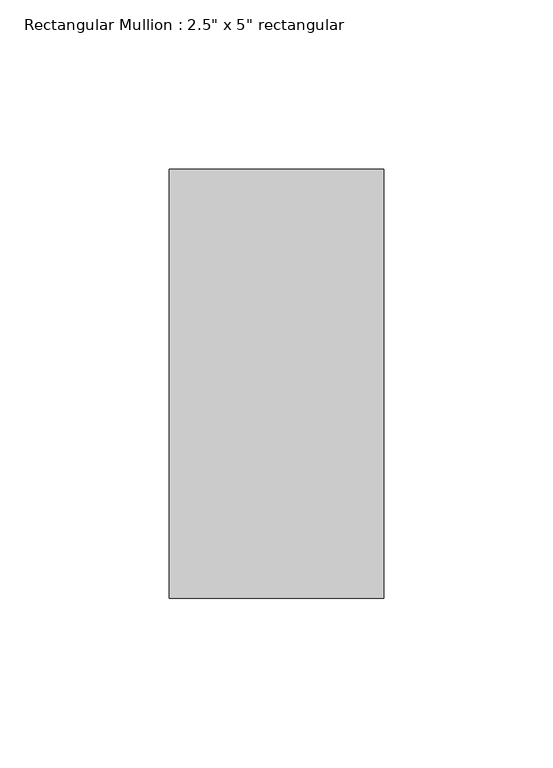
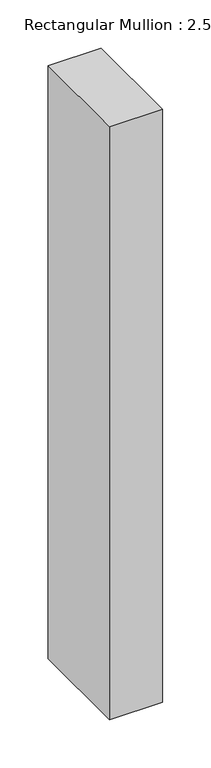
"""IFC4 building model written with IfcOpenShell, lengths in millimetres: member geometry."""

from ifc_helpers import new_model, si_unit, frame, origin, place, context, project, spatial, polyline, outline, extrude, source, transform, mapped, element, save


def member_424e4c0f(model_context):
    return source(origin(), model_context, "Body", "SweptSolid", [
        extrude(outline(polyline([(31.75, 63.5), (31.75, -63.5), (-31.75, -63.5), (-31.75, 63.5), (31.75, 63.5)])), frame((0.0, 0.0, -749.3168761), z_axis=(0.0, 0.0, 1.0), x_axis=(1.0, 0.0, 0.0)), (0.0, 0.0, 1.0), 749.3168761),
    ])


if __name__ == "__main__":
    model = new_model("IFC4")
    model_context = context("Model", 3, world=origin())
    ifc_project = project(units=[si_unit("LENGTHUNIT", "METRE", prefix="MILLI")], contexts=[model_context])
    site = spatial("IfcSite", under=ifc_project)
    building = spatial("IfcBuilding", under=site)
    placement = place(None, origin())
    member_shape = member_424e4c0f(model_context)
    element("IfcMember", 1, ObjectType="Rectangular Mullion : 2.5\" x 5\" rectangular", at=placement, inside=building, context=model_context, shape_type="MappedRepresentation", body=[
        mapped(member_shape, transform((0.0, 0.0, 0.0), x_axis=(1.0, 0.0, 0.0), y_axis=(0.0, 1.0, 0.0), z_axis=(0.0, 0.0, 1.0))),
    ])
    save(model, "model.ifc")

# Revit data of these elements
# Type "Rectangular Mullion : 2.5\" x 5\" rectangular"
#   built-in parameter 1007304 = 0.416667 (stored number, unit not read)
#   built-in parameter 1007301 = 0.104167 (stored number, unit not read)
#   built-in parameter 1007300 = 0.104167 (stored number, unit not read)
# Element 1 (IfcMember, "Rectangular Mullion : 2.5\" x 5\" rectangular")
#   Materials on its faces: "Aluminum"
# Materials
#   "Aluminum": class "Metal", colour RGB 247 247 247, transparency 0, Description = "Aluminum 6061", Cost = 0
